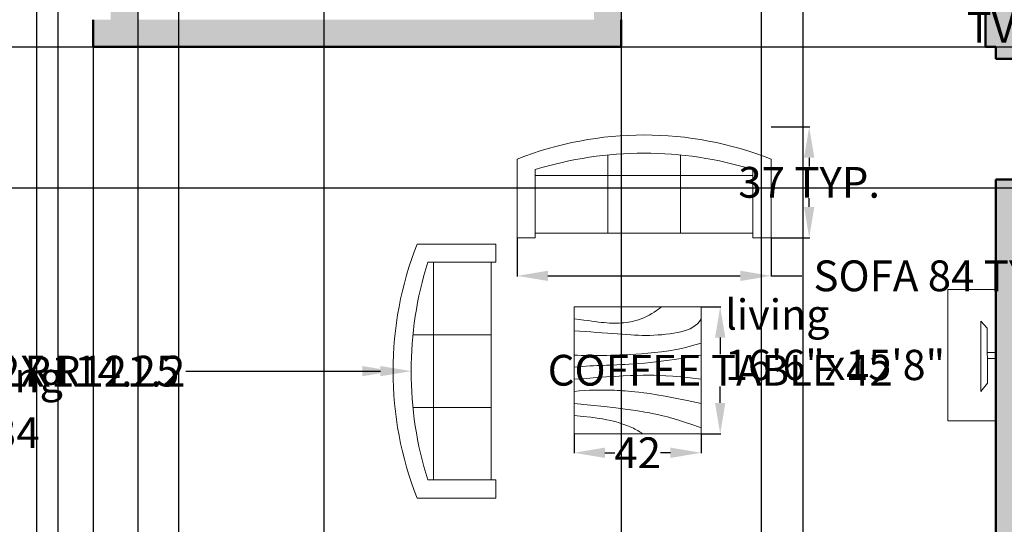
# Model space of a CAD drawing. Units: inches. Extents: x 12496 to 13538, y 6171 to 6892.
# Tile 4 of 6: x 12841 to 13167, y 6405 to 6572. Entities that reach past the tile are written whole.
import ezdxf

# ---------------------------------------------------------------- set-up
doc = ezdxf.new("R2010")
doc.units = ezdxf.units.IN
doc.header["$MEASUREMENT"] = 0
for name, color, linetype, lineweight in [('A-ANNO-DIMS', 2, 'Continuous', 18), ('A-AREA-IDEN', 7, 'Continuous', 25), ('A-FURN', 8, 'Continuous', 18), ('A-WALL', 7, 'Continuous', 50)]:
    doc.layers.add(name, color=color, linetype=linetype, lineweight=lineweight)
doc.layers.add('A-WALL-PATT', color=18, linetype='Continuous', lineweight=13, true_color=0x000000)
doc.styles.get("Standard").update_dxf_attribs({"font": 'arial.ttf'})
doc.dimstyles.get("Standard").update_dxf_attribs({"dimtxt": 10.18, "dimasz": 10.18, "dimexe": 0.18, "dimexo": 0.0625, "dimgap": 0.09, "dimtad": 0, "dimtih": 1, "dimtoh": 1, "dimdec": 0, "dimzin": 0, "dimdsep": 46, "dimlunit": 3, "dimtxsty": 'Standard', "dimcen": 0.09, "dimadec": 0, "dimazin": 0, "dimtfac": 1, "dimtdec": 0, "dimtofl": 0, "dimtmove": 0, "dimatfit": 3, "dimfxl": 1, "dimtolj": 1, "dimtzin": 0, "dimarcsym": 0})

# ---------------------------------------------------------------- blocks, each defined once
blk = doc.blocks.new('Sofa - Roundback 7 ft.')
for p, q in [((-12.00002, -32.4421), (-12.00003, -6.5971)), ((11.99997, -32.4421), (11.99998, -6.5971)), ((-36.000027, -34), (-36.000027, -11.4696)), ((35.99998, -34), (35.99998, -11.4696)), ((-35.999844, -13.3819), (35.9998, -13.3819)), ((-36.000027, -32.4421), (35.99998, -32.4421))]:
    blk.add_line(p, q)
for points in [[(-36.000027, -34), (-42.000027, -34), (-42.000027, -8)], [(41.99998, -8), (41.99998, -34), (35.99998, -34)]]:
    blk.add_lwpolyline(points)
for centre, radius, start, end in [((0, -114.25), 114.25, 68.43141, 111.5686), ((-0.00001, -127.1968), 121.1968, 72.72033, 107.2797)]:
    blk.add_arc(centre, radius, start, end)
blk = doc.blocks.new('Table - Square Woodgrain 42 x 42 in.')
blk.add_line((0, -42), (42, -42))
for points in [[(0, -4), (1.704, -4.2172), (3.2358, -4.4188), (4.615, -4.604), (5.8615, -4.7721), (6.9951, -4.9224), (8.0357, -5.0541), (9.0031, -5.1667), (9.9171, -5.2594), (10.7951, -5.3316), (11.6445, -5.3836), (12.4702, -5.4157), (13.277, -5.4283), (14.0698, -5.4217), (14.8535, -5.3964), (15.6331, -5.3526), (16.4133, -5.2908), (17.1986, -5.2103), (17.9913, -5.1062), (18.793, -4.9727), (19.6056, -4.8038), (20.4307, -4.5937), (21.2701, -4.3365), (22.1256, -4.0262), (22.9989, -3.6571), (23.888, -3.2272), (24.7756, -2.7516), (25.6408, -2.2491), (26.4624, -1.7387), (27.2195, -1.2395), (27.891, -0.7703), (28.456, -0.3501), (28.8934, 0.002)], [(0, -42), (0, 0), (42, 0), (42, -42)], [(0, -8), (1.8203, -8.1001), (3.6741, -8.2149), (5.5411, -8.3408), (7.4011, -8.4741), (9.2339, -8.6112), (11.0193, -8.7484), (12.7371, -8.8821), (14.3671, -9.0086), (15.8954, -9.1246), (17.3337, -9.2278), (18.6997, -9.3159), (20.0116, -9.387), (21.2871, -9.4389), (22.5442, -9.4696), (23.8008, -9.477), (25.0749, -9.459), (26.3791, -9.4137), (27.7049, -9.3403), (29.0383, -9.2382), (30.3655, -9.1068), (31.6728, -8.9455), (32.9461, -8.7535), (34.1717, -8.5304), (35.3358, -8.2756), (36.4268, -7.9863), (37.443, -7.6521), (38.3849, -7.2603), (39.253, -6.7986), (40.048, -6.2542), (40.7705, -5.6147), (41.421, -4.8674), (42, -4)], [(42, -12), (39.1784, -12.8621), (36.4519, -13.5654), (33.8246, -14.1294), (31.3004, -14.5731), (28.8832, -14.9161), (26.577, -15.1775), (24.3858, -15.3768), (22.3136, -15.5332), (20.3622, -15.6632), (18.5254, -15.7718), (16.7947, -15.8612), (15.1618, -15.9338), (13.6183, -15.9916), (12.1558, -16.0369), (10.7659, -16.0718), (9.4403, -16.0987), (8.1703, -16.1191), (6.9461, -16.1325), (5.7577, -16.1377), (4.595, -16.1335), (3.4479, -16.1188), (2.3064, -16.0924), (1.1604, -16.0532), (0, -16)], [(42, -16), (37.6529, -16.7365), (33.8802, -17.329), (30.6179, -17.7961), (27.8015, -18.1561), (25.3668, -18.4275), (23.2497, -18.6288), (21.3859, -18.7785), (19.7111, -18.8949), (18.1693, -18.9939), (16.7375, -19.0795), (15.401, -19.1534), (14.1449, -19.217), (12.9544, -19.2717), (11.8148, -19.3191), (10.7113, -19.3606), (9.6291, -19.3976), (8.5534, -19.4323), (7.47, -19.4689), (6.3643, -19.5122), (5.222, -19.5672), (4.0288, -19.6386), (2.7703, -19.7313), (1.4321, -19.8501), (0, -20)], [(0, -24), (3.9243, -23.6805), (7.4766, -23.4138), (10.6891, -23.1954), (13.5943, -23.0205), (16.2247, -22.8847), (18.6125, -22.7832), (20.7903, -22.7116), (22.7903, -22.6651), (24.6563, -22.642), (26.4764, -22.6507), (28.35, -22.7024), (30.3766, -22.8084), (32.6555, -22.98), (35.2861, -23.2283), (38.3678, -23.5645), (42, -24)], [(42, -32), (37.392, -31.017), (33.4585, -30.2231), (30.1291, -29.5949), (27.3334, -29.109), (25.0009, -28.742), (23.0612, -28.4707), (21.4439, -28.2716), (20.0786, -28.1215), (18.8998, -28.0002), (17.8609, -27.9014), (16.9206, -27.8219), (16.0371, -27.7588), (15.1691, -27.709), (14.2748, -27.6693), (13.3128, -27.6368), (12.2415, -27.6083), (11.0295, -27.5824), (9.6867, -27.5643), (8.233, -27.5608), (6.6884, -27.5787), (5.0728, -27.6248), (3.4062, -27.7058), (1.7086, -27.8286), (0, -28)], [(0, -32), (5.4026, -32.5358), (9.9494, -33.019), (13.7424, -33.4553), (16.8834, -33.8505), (19.4743, -34.2106), (21.6171, -34.5413), (23.4136, -34.8486), (24.9657, -35.1382), (26.3614, -35.4156), (27.6332, -35.6841), (28.7995, -35.9467), (29.8788, -36.2064), (30.8897, -36.4661), (31.8507, -36.7288), (32.7802, -36.9973), (33.6968, -37.2747), (34.6175, -37.5635), (35.5531, -37.8651), (36.5128, -38.1805), (37.506, -38.5108), (38.5421, -38.8568), (39.6302, -39.2197), (40.7797, -39.6004), (42, -40)], [(0, -36), (3.0098, -36.2857), (5.5354, -36.5643), (7.6368, -36.8359), (9.374, -37.1009), (10.807, -37.3597), (11.9957, -37.6126), (13.0002, -37.8599), (13.8804, -38.102), (14.6874, -38.3393), (15.4365, -38.5729), (16.1338, -38.8041), (16.7858, -39.0341), (17.3987, -39.264), (17.9787, -39.4952), (18.5322, -39.7288), (19.0655, -39.9662), (19.5832, -40.2081), (20.0842, -40.4544), (20.5657, -40.7046), (21.0249, -40.9581), (21.459, -41.2144), (21.8653, -41.4731), (22.2409, -41.7335), (22.5831, -41.9951)]]:
    blk.add_lwpolyline(points)
blk = doc.blocks.new('TV-CONSOLE')
for p, q in [((10.88, 32.95), (10.88, 9.78)), ((10.88, 32.95), (12.91, 30.72)), ((12.91, 30.72), (13.04, 12.51)), ((12.98, 22.62), (15.84, 22.62)), ((12.98, 20.62), (15.84, 20.62)), ((10.88, 9.78), (13.04, 12.51))]:
    blk.add_line(p, q)
blk.add_lwpolyline([(15.84, 43.51), (0, 43.51), (0, 0), (15.84, 0)], close=True)
blk = doc.blocks.new('*D29')
at = {"layer": 'A-ANNO-DIMS', "color": 0, "lineweight": -2, "transparency": 16777216}
for p, q in [((13303.55, 6569.73), (13293.37, 6569.73)), ((13303.55, 6563.27), (13303.55, 6569.91)), ((13336.87, 6569.73), (13313.73, 6569.73)), ((13347.05, 6563.27), (13347.05, 6569.91))]:
    blk.add_line(p, q, dxfattribs=at)
at = {"layer": 'A-ANNO-DIMS', "color": 0, "transparency": 16777216}
for points in [[(13313.73, 6571.43), (13313.73, 6568.03), (13303.55, 6569.73)], [(13336.87, 6571.43), (13336.87, 6568.03), (13347.05, 6569.73)]]:
    blk.add_solid(points, dxfattribs=at)
at = {"layer": 'Defpoints', "color": 0, "transparency": 16777216}
for p in [(13303.55, 6569.73), (13303.55, 6563.2), (13347.05, 6563.2)]:
    blk.add_point(p, dxfattribs=at)
at = {"layer": 'A-ANNO-DIMS', "color": 0, "transparency": 16777216, "insert": (13220.56, 6569.73), "char_height": 10.18, "attachment_point": 5}
blk.add_mtext('\\A1;TV CONSOLE 44 TYP.', dxfattribs=at)
blk = doc.blocks.new('*D43')
at = {"layer": 'A-ANNO-DIMS', "color": 0, "lineweight": -2, "transparency": 16777216}
for p, q in [((13005.46, 6500.01), (13005.46, 6487.3)), ((13089.46, 6500.01), (13089.46, 6487.3)), ((13015.64, 6487.48), (13079.28, 6487.48)), ((13089.46, 6487.48), (13099.64, 6487.48))]:
    blk.add_line(p, q, dxfattribs=at)
at = {"layer": 'A-ANNO-DIMS', "color": 0, "transparency": 16777216}
for points in [[(13015.64, 6489.17), (13015.64, 6485.78), (13005.46, 6487.48)], [(13079.28, 6489.17), (13079.28, 6485.78), (13089.46, 6487.48)]]:
    blk.add_solid(points, dxfattribs=at)
at = {"layer": 'Defpoints', "color": 0, "transparency": 16777216}
for p in [(13005.46, 6500.08), (13089.46, 6500.08), (13089.46, 6487.48)]:
    blk.add_point(p, dxfattribs=at)
at = {"layer": 'A-ANNO-DIMS', "color": 0, "transparency": 16777216, "insert": (13145.82, 6487.48), "char_height": 10.18, "attachment_point": 5}
blk.add_mtext('\\A1;SOFA 84 TYP.', dxfattribs=at)
blk = doc.blocks.new('*D44')
at = {"layer": 'A-ANNO-DIMS', "color": 0, "lineweight": -2, "transparency": 16777216}
for p, q in [((13089.53, 6536.74), (13102.24, 6536.74)), ((13102.06, 6526.56), (13102.06, 6523.7)), ((13102.06, 6510.26), (13102.06, 6513.12)), ((13089.53, 6500.08), (13102.24, 6500.08))]:
    blk.add_line(p, q, dxfattribs=at)
at = {"layer": 'A-ANNO-DIMS', "color": 0, "transparency": 16777216}
for points in [[(13100.37, 6526.56), (13103.76, 6526.56), (13102.06, 6536.74)], [(13100.37, 6510.26), (13103.76, 6510.26), (13102.06, 6500.08)]]:
    blk.add_solid(points, dxfattribs=at)
at = {"layer": 'Defpoints', "color": 0, "transparency": 16777216}
for p in [(13089.46, 6536.74), (13102.06, 6536.74), (13089.46, 6500.08)]:
    blk.add_point(p, dxfattribs=at)
at = {"layer": 'A-ANNO-DIMS', "color": 0, "transparency": 16777216, "insert": (13102.06, 6518.41), "char_height": 10.18, "attachment_point": 5}
blk.add_mtext('\\A1;37 TYP.', dxfattribs=at)
blk = doc.blocks.new('*D53')
at = {"layer": 'A-ANNO-DIMS', "color": 0, "lineweight": -2, "transparency": 16777216}
for p, q in [((13066.39, 6477.26), (13072.81, 6477.26)), ((13072.63, 6467.08), (13072.63, 6461.62)), ((13072.63, 6445.44), (13072.63, 6450.9)), ((13066.39, 6435.26), (13072.81, 6435.26))]:
    blk.add_line(p, q, dxfattribs=at)
at = {"layer": 'A-ANNO-DIMS', "color": 0, "transparency": 16777216}
for points in [[(13070.93, 6467.08), (13074.33, 6467.08), (13072.63, 6477.26)], [(13070.93, 6445.44), (13074.33, 6445.44), (13072.63, 6435.26)]]:
    blk.add_solid(points, dxfattribs=at)
at = {"layer": 'Defpoints', "color": 0, "transparency": 16777216}
for p in [(13066.33, 6477.26), (13072.63, 6477.26), (13066.33, 6435.26)]:
    blk.add_point(p, dxfattribs=at)
at = {"layer": 'A-ANNO-DIMS', "color": 0, "transparency": 16777216, "insert": (13072.63, 6456.26), "char_height": 10.18, "attachment_point": 5}
blk.add_mtext('\\A1;COFFEE TABLE 42', dxfattribs=at)
blk = doc.blocks.new('*D54')
at = {"layer": 'A-ANNO-DIMS', "color": 0, "lineweight": -2, "transparency": 16777216}
for p, q in [((13024.33, 6435.2), (13024.33, 6428.78)), ((13066.33, 6435.2), (13066.33, 6428.78)), ((13034.51, 6428.96), (13037.79, 6428.96)), ((13056.15, 6428.96), (13052.86, 6428.96))]:
    blk.add_line(p, q, dxfattribs=at)
at = {"layer": 'A-ANNO-DIMS', "color": 0, "transparency": 16777216}
for points in [[(13034.51, 6430.66), (13034.51, 6427.26), (13024.33, 6428.96)], [(13056.15, 6430.66), (13056.15, 6427.26), (13066.33, 6428.96)]]:
    blk.add_solid(points, dxfattribs=at)
at = {"layer": 'Defpoints', "color": 0, "transparency": 16777216}
for p in [(13024.33, 6435.26), (13066.33, 6435.26), (13066.33, 6428.96)]:
    blk.add_point(p, dxfattribs=at)
at = {"layer": 'A-ANNO-DIMS', "color": 0, "transparency": 16777216, "insert": (13045.33, 6428.96), "char_height": 10.18, "attachment_point": 5}
blk.add_mtext('\\A1;42', dxfattribs=at)
blk = doc.blocks.new('*D66')
at = {"layer": 'A-ANNO-DIMS', "color": 0, "lineweight": -2, "transparency": 16777216}
for p, q in [((12846.6, 6312.58), (12846.6, 6885.67)), ((12856.78, 6885.49), (12955.96, 6885.49)), ((13089.92, 6885.49), (12990.74, 6885.49)), ((13100.1, 6312.58), (13100.1, 6885.67))]:
    blk.add_line(p, q, dxfattribs=at)
at = {"layer": 'A-ANNO-DIMS', "color": 0, "transparency": 16777216}
for points in [[(12856.78, 6887.18), (12856.78, 6883.79), (12846.6, 6885.49)], [(13089.92, 6887.18), (13089.92, 6883.79), (13100.1, 6885.49)]]:
    blk.add_solid(points, dxfattribs=at)
at = {"layer": 'Defpoints', "color": 0, "transparency": 16777216}
for p in [(13100.1, 6885.49), (12846.6, 6312.52), (13100.1, 6312.52)]:
    blk.add_point(p, dxfattribs=at)
at = {"layer": 'A-ANNO-DIMS', "color": 0, "transparency": 16777216, "insert": (12973.35, 6885.49), "char_height": 10.18, "attachment_point": 5}
blk.add_mtext('\\A1;253.5', dxfattribs=at)
blk = doc.blocks.new('*D76')
at = {"layer": 'A-ANNO-DIMS', "color": 0, "lineweight": -2, "transparency": 16777216}
for p, q in [((12721.51, 6563.2), (13486.8, 6563.2)), ((13486.62, 6553.02), (13486.62, 6545.16)), ((13486.62, 6526.72), (13486.62, 6534.58)), ((12721.51, 6516.54), (13486.8, 6516.54))]:
    blk.add_line(p, q, dxfattribs=at)
at = {"layer": 'A-ANNO-DIMS', "color": 0, "transparency": 16777216}
for points in [[(13484.92, 6553.02), (13488.32, 6553.02), (13486.62, 6563.2)], [(13484.92, 6526.72), (13488.32, 6526.72), (13486.62, 6516.54)]]:
    blk.add_solid(points, dxfattribs=at)
at = {"layer": 'Defpoints', "color": 0, "transparency": 16777216}
for p in [(12721.45, 6563.2), (13486.62, 6563.2), (12721.45, 6516.54)]:
    blk.add_point(p, dxfattribs=at)
at = {"layer": 'A-ANNO-DIMS', "color": 0, "transparency": 16777216, "insert": (13486.62, 6539.87), "char_height": 10.18, "attachment_point": 5}
blk.add_mtext('\\A1;46.67', dxfattribs=at)
blk = doc.blocks.new('*D81')
at = {"layer": 'A-ANNO-DIMS', "color": 0, "lineweight": -2, "transparency": 16777216}
for p, q in [((12880.07, 6781.83), (12880.07, 6177.12)), ((12941.5, 6781.83), (12941.5, 6177.12)), ((12890.25, 6177.3), (12893.54, 6177.3)), ((12931.32, 6177.3), (12928.02, 6177.3))]:
    blk.add_line(p, q, dxfattribs=at)
at = {"layer": 'A-ANNO-DIMS', "color": 0, "transparency": 16777216}
for points in [[(12890.25, 6179), (12890.25, 6175.6), (12880.07, 6177.3)], [(12931.32, 6179), (12931.32, 6175.6), (12941.5, 6177.3)]]:
    blk.add_solid(points, dxfattribs=at)
at = {"layer": 'Defpoints', "color": 0, "transparency": 16777216}
for p in [(12880.07, 6781.89), (12941.5, 6781.89), (12941.5, 6177.3)]:
    blk.add_point(p, dxfattribs=at)
at = {"layer": 'A-ANNO-DIMS', "color": 0, "transparency": 16777216, "insert": (12910.78, 6177.3), "char_height": 10.18, "attachment_point": 5}
blk.add_mtext('\\A1;61.42', dxfattribs=at)
blk = doc.blocks.new('*D82')
at = {"layer": 'A-ANNO-DIMS', "color": 0, "lineweight": -2, "transparency": 16777216}
for p, q in [((13039.92, 6781.83), (13039.92, 6177.12)), ((13086.15, 6781.83), (13086.15, 6177.12)), ((13029.74, 6177.3), (13019.56, 6177.3)), ((13096.33, 6177.3), (13106.51, 6177.3))]:
    blk.add_line(p, q, dxfattribs=at)
at = {"layer": 'A-ANNO-DIMS', "color": 0, "transparency": 16777216}
for points in [[(13029.74, 6179), (13029.74, 6175.6), (13039.92, 6177.3)], [(13096.33, 6179), (13096.33, 6175.6), (13086.15, 6177.3)]]:
    blk.add_solid(points, dxfattribs=at)
at = {"layer": 'Defpoints', "color": 0, "transparency": 16777216}
for p in [(13039.92, 6781.89), (13086.15, 6781.89), (13086.15, 6177.3)]:
    blk.add_point(p, dxfattribs=at)
at = {"layer": 'A-ANNO-DIMS', "color": 0, "transparency": 16777216, "insert": (13063.03, 6177.3), "char_height": 10.18, "attachment_point": 5}
blk.add_mtext('\\A1;46.23', dxfattribs=at)
blk = doc.blocks.new('*D84')
at = {"layer": 'A-ANNO-DIMS', "color": 0, "lineweight": -2, "transparency": 16777216}
for p, q in [((12853.64, 6312.58), (12853.64, 6885.67)), ((12863.82, 6885.49), (12866.07, 6885.49)), ((12883.46, 6885.49), (12881.21, 6885.49)), ((12893.64, 6312.58), (12893.64, 6885.67))]:
    blk.add_line(p, q, dxfattribs=at)
at = {"layer": 'A-ANNO-DIMS', "color": 0, "transparency": 16777216}
for points in [[(12863.82, 6887.18), (12863.82, 6883.79), (12853.64, 6885.49)], [(12883.46, 6887.18), (12883.46, 6883.79), (12893.64, 6885.49)]]:
    blk.add_solid(points, dxfattribs=at)
at = {"layer": 'Defpoints', "color": 0, "transparency": 16777216}
for p in [(12893.64, 6885.49), (12853.64, 6312.52), (12893.64, 6312.52)]:
    blk.add_point(p, dxfattribs=at)
at = {"layer": 'A-ANNO-DIMS', "color": 0, "transparency": 16777216, "insert": (12873.64, 6885.49), "char_height": 10.18, "attachment_point": 5}
blk.add_mtext('\\A1;40', dxfattribs=at)
blk = doc.blocks.new('*D87')
at = {"layer": 'A-ANNO-DIMS', "color": 0, "lineweight": -2, "transparency": 16777216}
for p, q in [((12825.27, 6572.14), (12825.27, 6177.12)), ((12865.27, 6572.14), (12865.27, 6177.12)), ((12835.45, 6177.3), (12837.7, 6177.3)), ((12855.09, 6177.3), (12852.83, 6177.3))]:
    blk.add_line(p, q, dxfattribs=at)
at = {"layer": 'A-ANNO-DIMS', "color": 0, "transparency": 16777216}
for points in [[(12835.45, 6179), (12835.45, 6175.6), (12825.27, 6177.3)], [(12855.09, 6179), (12855.09, 6175.6), (12865.27, 6177.3)]]:
    blk.add_solid(points, dxfattribs=at)
at = {"layer": 'Defpoints', "color": 0, "transparency": 16777216}
for p in [(12825.27, 6572.2), (12865.27, 6572.2), (12865.27, 6177.3)]:
    blk.add_point(p, dxfattribs=at)
at = {"layer": 'A-ANNO-DIMS', "color": 0, "transparency": 16777216, "insert": (12845.27, 6177.3), "char_height": 10.18, "attachment_point": 5}
blk.add_mtext('\\A1;40', dxfattribs=at)
blk = doc.blocks.new('*D88')
at = {"layer": 'A-ANNO-DIMS', "color": 0, "lineweight": -2, "transparency": 16777216}
for p, q in [((12782.49, 6435.61), (12775.28, 6428.42)), ((12792.67, 6435.61), (12782.49, 6435.61)), ((12761.24, 6414.51), (12761.42, 6414.51)), ((12761.33, 6414.42), (12761.33, 6414.6))]:
    blk.add_line(p, q, dxfattribs=at)
at = {"layer": 'A-ANNO-DIMS', "color": 0, "transparency": 16777216}
blk.add_solid([(12774.08, 6429.62), (12776.48, 6427.22), (12768.07, 6421.23)], dxfattribs=at)
at = {"layer": 'Defpoints', "color": 0, "transparency": 16777216}
for p in [(12768.07, 6421.23), (12754.59, 6407.79)]:
    blk.add_point(p, dxfattribs=at)
at = {"layer": 'A-ANNO-DIMS', "color": 0, "transparency": 16777216, "insert": (12819.41, 6435.61), "char_height": 10.18, "attachment_point": 5}
blk.add_mtext('\\A1;∅19.034', dxfattribs=at)
blk = doc.blocks.new('*D89')
at = {"layer": 'A-ANNO-DIMS', "color": 0, "lineweight": -2, "transparency": 16777216}
for p, q in [((12897.7, 6455.96), (12960.24, 6455.96)), ((13091.53, 6455.96), (13091.71, 6455.96)), ((13091.62, 6455.87), (13091.62, 6456.05))]:
    blk.add_line(p, q, dxfattribs=at)
at = {"layer": 'A-ANNO-DIMS', "color": 0, "transparency": 16777216}
blk.add_solid([(12960.24, 6457.66), (12960.24, 6454.26), (12970.42, 6455.96)], dxfattribs=at)
at = {"layer": 'Defpoints', "color": 0, "transparency": 16777216}
for p in [(12970.42, 6455.96), (13091.62, 6455.96)]:
    blk.add_point(p, dxfattribs=at)
at = {"layer": 'A-ANNO-DIMS', "color": 0, "transparency": 16777216, "insert": (12864.59, 6455.96), "char_height": 10.18, "attachment_point": 5}
blk.add_mtext('\\A1;2X R121.2', dxfattribs=at)
blk = doc.blocks.new('*D90')
at = {"layer": 'A-ANNO-DIMS', "color": 0, "lineweight": -2, "transparency": 16777216}
for p, q in [((12895.87, 6455.96), (12954.24, 6455.96)), ((13078.58, 6455.96), (13078.76, 6455.96)), ((13078.67, 6455.87), (13078.67, 6456.05))]:
    blk.add_line(p, q, dxfattribs=at)
at = {"layer": 'A-ANNO-DIMS', "color": 0, "transparency": 16777216}
blk.add_solid([(12954.24, 6457.66), (12954.24, 6454.26), (12964.42, 6455.96)], dxfattribs=at)
at = {"layer": 'Defpoints', "color": 0, "transparency": 16777216}
for p in [(12964.42, 6455.96), (13078.67, 6455.96)]:
    blk.add_point(p, dxfattribs=at)
at = {"layer": 'A-ANNO-DIMS', "color": 0, "transparency": 16777216, "insert": (12858.72, 6455.96), "char_height": 10.18, "attachment_point": 5}
blk.add_mtext('\\A1;2X R114.25', dxfattribs=at)

msp = doc.modelspace()

# ---------------------------------------------------------------- hatches: boundary and pattern name
at = {"layer": 'A-WALL-PATT'}
h = msp.add_hatch(color=256, dxfattribs=at)
h.dxf.hatch_style = 1
h.paths.add_polyline_path([(13443.0285, 6790.8943), (13327.7025, 6790.8943), (13327.7025, 6781.8943), (13434.0285, 6781.8943), (13434.0285, 6572.2028), (13169.3765, 6572.2028), (13169.3765, 6576.9323), (13160.3765, 6576.9323), (13160.3765, 6563.2028), (13163.811, 6563.2028), (13163.811, 6559.305), (13172.811, 6559.305), (13172.811, 6563.2028), (13434.0285, 6563.2028), (13434.0285, 6402.794), (13331.4198, 6402.794), (13331.4198, 6393.8103), (13434.0285, 6393.8103), (13434.0285, 6220.8943), (13443.0285, 6220.8943)])
h.paths.add_polyline_path([(13172.811, 6519.305), (13163.811, 6519.305), (13163.811, 6402.8103), (12944.6655, 6402.8103), (12944.6655, 6393.8103), (13100.0985, 6393.8103), (13100.0985, 6312.5223), (13035.7682, 6312.5223), (13035.7682, 6303.5223), (13109.0985, 6303.5223), (13109.0985, 6393.8103), (13279.4198, 6393.8103), (13279.4198, 6402.8103), (13172.811, 6402.8103)])
h.paths.add_polyline_path([(13109.0985, 6229.8943), (12846.603, 6229.8943), (12846.603, 6303.5223), (12853.6371, 6303.5223), (12853.6371, 6312.5223), (12846.603, 6312.5223), (12846.603, 6393.8103), (12872.7237, 6393.8103), (12872.7237, 6402.8103), (12846.603, 6402.8103), (12837.603, 6402.8103), (12837.603, 6229.8943), (12760.3881, 6229.8943), (12760.3881, 6220.8943), (13109.0985, 6220.8943)])
h.paths.add_polyline_path([(12708.3881, 6229.8943), (12631.1731, 6229.8943), (12631.1731, 6336.5598), (12702.8967, 6336.5598), (12702.8967, 6345.5598), (12631.1731, 6345.5598), (12631.1731, 6355.6851), (12622.1731, 6355.6851), (12622.1731, 6220.8943), (12708.3881, 6220.8943)])
h.paths.add_polyline_path([(12743.3881, 6402.8103), (12631.1731, 6402.8103), (12631.1731, 6523.6486), (12622.1731, 6523.6486), (12622.1731, 6383.6851), (12631.1731, 6383.6851), (12631.1731, 6393.8103), (12734.3881, 6393.8103), (12734.3881, 6345.5598), (12731.8151, 6345.5598), (12731.8151, 6336.5598), (12734.3881, 6336.5598), (12743.3881, 6336.5598)])
h.paths.add_polyline_path([(13039.9206, 6572.2028), (13039.9206, 6638.8628), (13048.7069, 6638.8628), (13048.7069, 6647.8628), (13039.9206, 6647.8628), (12930.9211, 6647.8628), (12930.9211, 6638.8628), (13030.9206, 6638.8628), (13030.9206, 6572.2028), (12880.0706, 6572.2028), (12880.0706, 6576.9323), (12871.0706, 6576.9323), (12871.0706, 6572.2028), (12865.2657, 6572.2028), (12865.2657, 6563.2028), (13039.9206, 6563.2028)])
h.paths.add_polyline_path([(13039.9206, 6781.8943), (13086.1485, 6781.8943), (13086.1485, 6790.8943), (12969.4956, 6790.8943), (12969.4956, 6781.8943), (13030.9206, 6781.8943), (13030.9206, 6647.8628), (13039.9206, 6647.8628)])
h.paths.add_polyline_path([(13169.3765, 6781.8943), (13275.7025, 6781.8943), (13275.7025, 6790.8943), (13114.1485, 6790.8943), (13114.1485, 6781.8943), (13160.3765, 6781.8943), (13160.3765, 6647.8628), (13088.7069, 6647.8628), (13088.7069, 6638.8628), (13160.3765, 6638.8628), (13160.3765, 6616.9323), (13169.3765, 6616.9323)])

# ---------------------------------------------------------------- linework, layer by layer
at = {"layer": 'A-WALL'}
for p, q in [((13160.3765, 6563.2028), (13160.3765, 6576.9323)), ((12865.2657, 6572.2028), (12865.2657, 6563.2028)), ((13039.9206, 6563.2028), (13039.9206, 6572.2028)), ((12865.2657, 6563.2028), (13039.9206, 6563.2028)), ((13160.3765, 6563.2028), (13163.811, 6563.2028)), ((13163.811, 6563.2028), (13163.811, 6559.305)), ((13172.811, 6559.305), (13163.811, 6559.305)), ((13172.811, 6519.305), (13163.811, 6519.305)), ((13163.811, 6519.305), (13163.811, 6402.8103))]:
    msp.add_line(p, q, dxfattribs=at)

# ---------------------------------------------------------------- block references
at = {"layer": 'A-FURN'}
for name, p in [('Sofa - Roundback 7 ft.', (13047.464, 6534.0764)), ('TV-CONSOLE', (13147.97, 6439.499)), ('Table - Square Woodgrain 42 x 42 in.', (13024.3288, 6477.2596))]:
    msp.add_blockref(name, p, dxfattribs=at)
at = {"layer": 'A-FURN', "rotation": 90}
msp.add_blockref('Sofa - Roundback 7 ft.', (12964.4203, 6455.9615), dxfattribs=at)

# ---------------------------------------------------------------- texts
at = {"layer": 'A-AREA-IDEN', "char_height": 10, "attachment_point": 1}
for s, insert in [('living\\P16\'6"x15\'8"', (13074.2732, 6479.6795)), ('dining', (12814.94, 6458.9326))]:
    msp.add_mtext_dynamic_manual_height_columns(s, width=261.947845, gutter_width=1, heights=[0], dxfattribs=dict(at, insert=insert))

# ---------------------------------------------------------------- dimensions: what is measured, and where the dimension line sits
at = {"layer": 'A-ANNO-DIMS'}
for base, p1, p2, override, picture, middle in [((13100.0985, 6885.4873), (12846.603, 6312.5223), (13100.0985, 6312.5223), {"dimdec": 1, "dimlfac": 1, "dimrnd": 0, "dimzin": 0, "dimdsep": 46, "dimlunit": 2}, '*D66', (12973.3508, 6885.4873)), ((12893.6371, 6885.4873), (12853.6371, 6312.5223), (12893.6371, 6312.5223), {"dimdec": 0, "dimlfac": 1, "dimrnd": 0, "dimzin": 0, "dimdsep": 46, "dimlunit": 2}, '*D84', (12873.6371, 6885.4873)), ((12941.49558, 6177.30135), (12880.07062, 6781.89435), (12941.49558, 6781.89435), {"dimdec": 2, "dimlfac": 1, "dimrnd": 0, "dimzin": 0, "dimdsep": 46, "dimlunit": 2}, '*D81', (12910.7831, 6177.30135)), ((13086.1485, 6177.3013), (13039.9206, 6781.8943), (13086.1485, 6781.8943), {"dimdec": 2, "dimlfac": 1, "dimrnd": 0, "dimzin": 0, "dimdsep": 46, "dimlunit": 2}, '*D82', (13063.0345, 6177.3013)), ((12865.2657, 6177.3013), (12825.2657, 6572.2028), (12865.2657, 6572.2028), {"dimdec": 0, "dimlfac": 1, "dimrnd": 0, "dimzin": 0, "dimdsep": 46, "dimlunit": 2}, '*D87', (12845.2657, 6177.3013)), ((13066.3288, 6428.9593), (13024.3288, 6435.2596), (13066.3288, 6435.2596), {"dimdec": 0, "dimlfac": 1, "dimrnd": 0, "dimzin": 0, "dimdsep": 46, "dimlunit": 2}, '*D54', (13045.3288, 6428.9593))]:
    dim = msp.add_linear_dim(base=base, p1=p1, p2=p2, dimstyle='Standard', override=override, dxfattribs=at)
    dim.commit()
    dim.dimension.update_dxf_attribs({"geometry": picture, "text_midpoint": middle})
for base, p1, p2, angle, text, picture, middle in [((13303.5465, 6569.729), (13347.0546, 6563.2028), (13303.5465, 6563.2028), 180, 'TV CONSOLE <> TYP.', '*D29', (13220.5618, 6569.729)), ((13102.0639, 6536.7431), (13089.4639, 6500.0764), (13089.4639, 6536.7431), 90, '<> TYP.', '*D44', (13102.0639, 6518.4098)), ((13072.6291, 6477.2616), (13066.3288, 6435.2596), (13066.3288, 6477.2616), 90, 'COFFEE TABLE <>', '*D53', (13072.6291, 6456.2606))]:
    dim = msp.add_linear_dim(base=base, p1=p1, p2=p2, angle=angle, text=text, dimstyle='Standard', override={"dimdec": 0, "dimlfac": 1, "dimrnd": 0, "dimzin": 0, "dimdsep": 46, "dimlunit": 2}, dxfattribs=at)
    dim.commit()
    dim.dimension.update_dxf_attribs({"geometry": picture, "text_midpoint": middle})
dim = msp.add_linear_dim(base=(13486.6215, 6563.2028), p1=(12721.4504, 6516.5354), p2=(12721.4504, 6563.2028), angle=90, dimstyle='Standard', override={"dimdec": 2, "dimlfac": 1, "dimrnd": 0, "dimzin": 0, "dimdsep": 46, "dimlunit": 2}, dxfattribs=at)
dim.commit()
dim.dimension.update_dxf_attribs({"geometry": '*D76', "text_midpoint": (13486.6215, 6539.8691)})
dim = msp.add_linear_dim(base=(13089.4639, 6487.4764), p1=(13005.4639, 6500.0764), p2=(13089.4639, 6500.0764), text='SOFA <> TYP.', dimstyle='Standard', override={"dimdec": 0, "dimlfac": 1, "dimrnd": 0, "dimzin": 0, "dimdsep": 46, "dimlunit": 2}, dxfattribs=at)
dim.commit()
dim.dimension.update_dxf_attribs({"geometry": '*D43', "text_midpoint": (13145.8217, 6487.4764)})
for center, mpoint, override, picture, middle in [((13078.6703, 6455.9615), (12964.4203, 6455.961), {"dimdec": 2, "dimlfac": 1, "dimrnd": 0, "dimzin": 0, "dimdsep": 46, "dimlunit": 2}, '*D90', (12895.8703, 6455.9607)), ((13091.6171, 6455.9615), (12970.4203, 6455.961), {"dimdec": 1, "dimlfac": 1, "dimrnd": 0, "dimzin": 0, "dimdsep": 46, "dimlunit": 2}, '*D89', (12897.7022, 6455.9607))]:
    dim = msp.add_radius_dim(center=center, mpoint=mpoint, text='2X <>', dimstyle='Standard', override=override, dxfattribs=at)
    dim.commit()
    dim.dimension.update_dxf_attribs({"geometry": picture, "text_midpoint": middle, "dimtype": 164})
dim = msp.add_diameter_dim_2p(p1=(12754.5938, 6407.7898), p2=(12768.0719, 6421.2297), dimstyle='Standard', override={"dimdec": 3, "dimlfac": 1, "dimrnd": 0, "dimzin": 0, "dimdsep": 46, "dimlunit": 2}, dxfattribs=at)
dim.commit()
dim.dimension.update_dxf_attribs({"geometry": '*D88', "text_midpoint": (12819.4068, 6435.606), "dimtype": 163})

doc.saveas('drawing.dxf')
